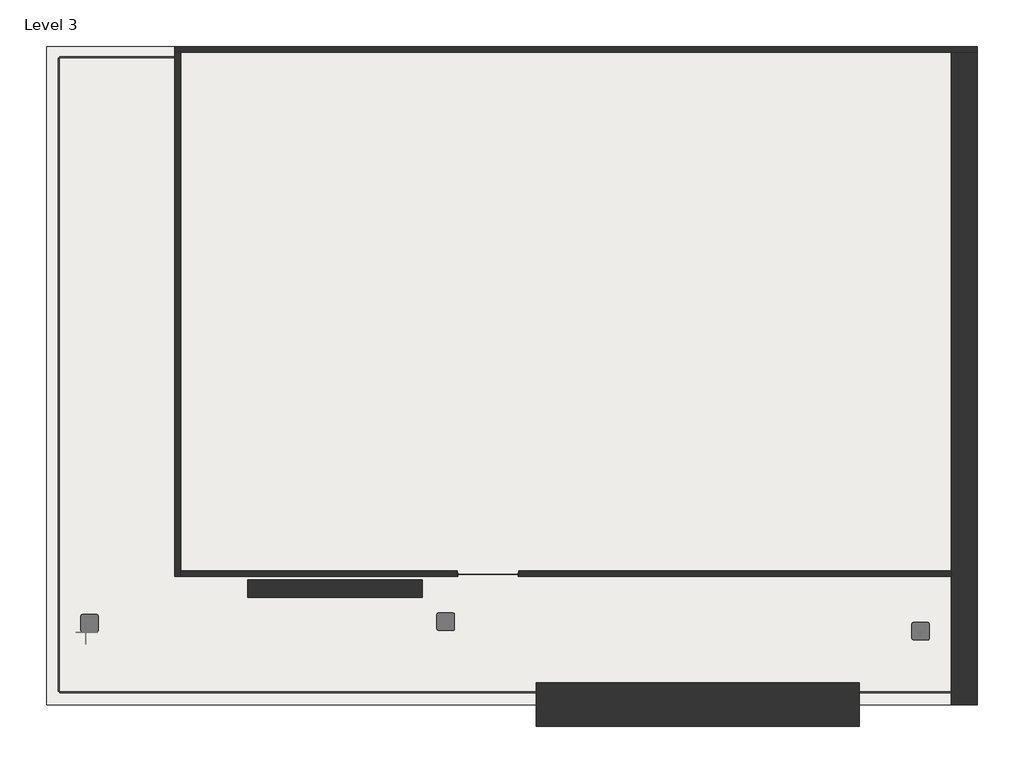
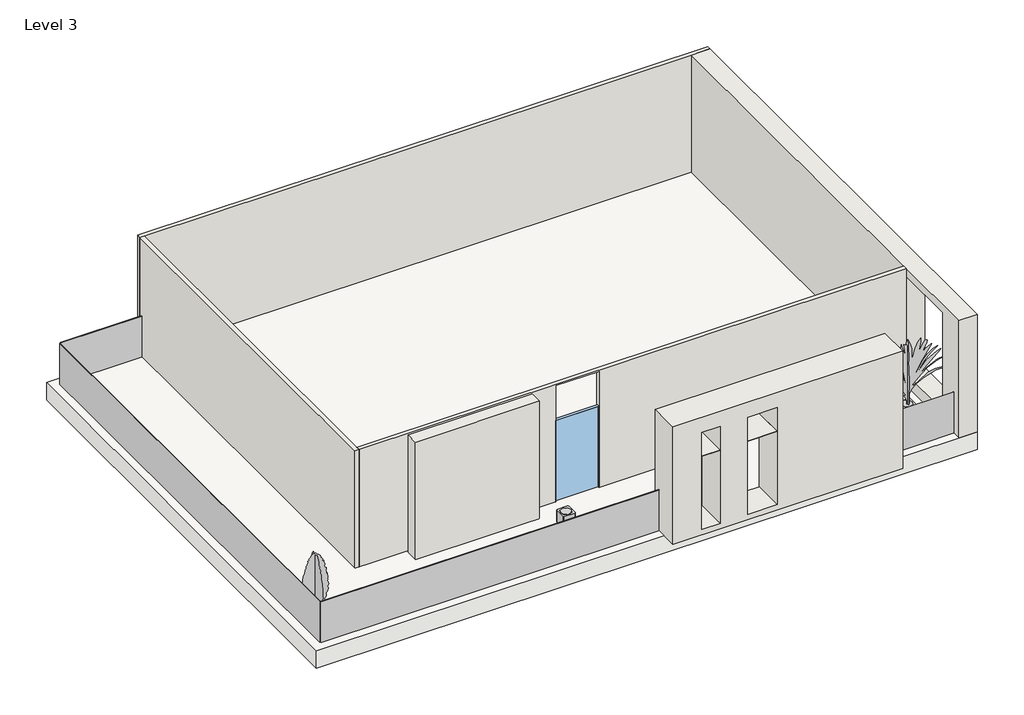
# One storey, incomplete: 6 walls, 4 plates, 3 proxies, 2 geographic elements, 1 slab, 1 window.
"""IFC4 building model written with IfcOpenShell, lengths in millimetres."""

from ifc_helpers import new_model, si_unit, frame, origin, place, context, project, spatial, polyline, outline, extrude, faceted_brep, transform, mapped, element, save
from components import proxy_13b82c07, rpc_tree_conifer_chinese_juniper_7_5155a079, rpc_tree_tropical_0177ab4a, system_panel_glazed_7ce5a3c2, system_panel_glazed_6867f845, system_panel_glazed_ba49168f, system_panel_glazed_c41ca4f4, window_2382273a

model = new_model("IFC4")

# Units and contexts
model_context = context("Model", 3, world=origin())
ifc_project = project(units=[si_unit("LENGTHUNIT", "METRE", prefix="MILLI")], contexts=[model_context])

# Site, building, storey
site = spatial("IfcSite", under=ifc_project)
building = spatial("IfcBuilding", under=site)
storey = spatial("IfcBuildingStorey", under=building, Name="Level 3", Elevation=6096.0)

# Proxies
placement = place(None, origin())
proxy_shape = proxy_13b82c07(model_context)
element("IfcBuildingElementProxy", 1, Name="Air Conditioner-Outside Unit : 33\" x 24\" x 24\"", ObjectType="Air Conditioner-Outside Unit : 33\" x 24\" x 24\"", at=placement, inside=storey, context=model_context, shape_type="MappedRepresentation", body=[
    mapped(proxy_shape, transform((-24603.5874719, -2613.1632813, 7010.4), x_axis=(1.0, 0.0, 0.0), y_axis=(0.0, 1.0, 0.0), z_axis=(0.0, 0.0, 1.0))),
])
element("IfcBuildingElementProxy", 2, Name="Air Conditioner-Outside Unit : 33\" x 24\" x 24\"", ObjectType="Air Conditioner-Outside Unit : 33\" x 24\" x 24\"", at=placement, inside=storey, context=model_context, shape_type="MappedRepresentation", body=[
    mapped(proxy_shape, transform((4377.8125281, -2892.5632813, 7010.4), x_axis=(1.0, 0.0, 0.0), y_axis=(0.0, 1.0, 0.0), z_axis=(0.0, 0.0, 1.0))),
])
element("IfcBuildingElementProxy", 3, Name="Air Conditioner-Outside Unit : 33\" x 24\" x 24\"", ObjectType="Air Conditioner-Outside Unit : 33\" x 24\" x 24\"", at=placement, inside=storey, context=model_context, shape_type="MappedRepresentation", body=[
    mapped(proxy_shape, transform((-12182.9874719, -2562.3632813, 7010.4), x_axis=(1.0, 0.0, 0.0), y_axis=(0.0, 1.0, 0.0), z_axis=(0.0, 0.0, 1.0))),
])

# Geographic elements
rpc_tree_conifer_chinese_juniper_7_shape = rpc_tree_conifer_chinese_juniper_7_5155a079(model_context)
element("IfcGeographicElement", 4, ObjectType="RPC Tree - Conifer : Chinese Juniper - 7'", at=placement, inside=storey, context=model_context, shape_type="MappedRepresentation", body=[
    mapped(rpc_tree_conifer_chinese_juniper_7_shape, transform((-24730.784143, -2943.3632813, 7010.4), x_axis=(1.0, 0.0, 0.0), y_axis=(0.0, 1.0, 0.0), z_axis=(0.0, 0.0, 1.0))),
])
rpc_tree_tropical_shape = rpc_tree_tropical_0177ab4a(model_context)
element("IfcGeographicElement", 5, ObjectType="RPC Tree - Tropical", at=placement, inside=storey, context=model_context, shape_type="MappedRepresentation", body=[
    mapped(rpc_tree_tropical_shape, transform((4377.8125281, -2943.3632813, 7010.4), x_axis=(1.0, 0.0, 0.0), y_axis=(0.0, 1.0, 0.0), z_axis=(0.0, 0.0, 1.0))),
])

# Plates
system_panel_glazed_shape = system_panel_glazed_7ce5a3c2(model_context)
element("IfcPlate", 6, ObjectType="System Panel : Glazed", at=placement, inside=storey, context=model_context, shape_type="MappedRepresentation", body=[
    mapped(system_panel_glazed_shape, transform((3844.4125281, -5000.7632813, 7010.4), x_axis=(-1.0, 0.0, 0.0), y_axis=(0.0, -1.0, 0.0), z_axis=(0.0, 0.0, 1.0))),
])
system_panel_glazed_2_shape = system_panel_glazed_6867f845(model_context)
element("IfcPlate", 7, ObjectType="System Panel : Glazed", at=placement, inside=storey, context=model_context, shape_type="MappedRepresentation", body=[
    mapped(system_panel_glazed_2_shape, transform((-17339.1874719, -5000.7632813, 7010.4), x_axis=(-1.0, 0.0, 0.0), y_axis=(0.0, -1.0, 0.0), z_axis=(0.0, 0.0, 1.0))),
])
system_panel_glazed_3_shape = system_panel_glazed_ba49168f(model_context)
element("IfcPlate", 8, ObjectType="System Panel : Glazed", at=placement, inside=storey, context=model_context, shape_type="MappedRepresentation", body=[
    mapped(system_panel_glazed_3_shape, transform((-25644.9874719, 6048.2367187, 7010.4), x_axis=(0.0, 1.0, 0.0), y_axis=(-1.0, 0.0, 0.0), z_axis=(0.0, 0.0, 1.0))),
])
system_panel_glazed_4_shape = system_panel_glazed_c41ca4f4(model_context)
element("IfcPlate", 9, ObjectType="System Panel : Glazed", at=placement, inside=storey, context=model_context, shape_type="MappedRepresentation", body=[
    mapped(system_panel_glazed_4_shape, transform((-23638.3874719, 17097.2367187, 7010.4), x_axis=(1.0, 0.0, 0.0), y_axis=(0.0, 1.0, 0.0), z_axis=(0.0, 0.0, 1.0))),
])

# Slab
element("IfcSlab", 10, ObjectType="Generic - 3'", at=placement, inside=storey, context=model_context, shape_type="SweptSolid", body=[
    extrude(outline(polyline([(-26102.1874719, -5457.9632813), (-26102.1874719, 17503.6367187), (6359.0125281, 17503.6367187), (6359.0125281, -5457.9632813), (-26102.1874719, -5457.9632813)])), frame((0.0, 0.0, 6096.0), z_axis=(0.0, 0.0, 1.0), x_axis=(1.0, 0.0, 0.0)), (0.0, 0.0, 1.0), 914.4),
])

# Walls
element("IfcWall", 11, ObjectType="Generic - 3'", at=placement, inside=storey, context=model_context, shape_type="Brep", body=[
    faceted_brep([(5444.6125281, 17300.4367187, 7010.4), (5444.6125281, -784.3632813, 7010.4), (5444.6125281, -987.5632813, 7010.4), (5444.6125281, -5457.9632813, 7010.4), (5444.6125281, -5457.9632813, 13106.4), (5444.6125281, -987.5632813, 13106.4), (5444.6125281, -784.3632813, 13106.4), (5444.6125281, 17300.4367187, 13106.4), (5444.6125281, -4035.5632813, 12658.887938), (5444.6125281, -4035.5632813, 7629.687938), (5444.6125281, -987.5632813, 7629.687938), (5444.6125281, -987.5632813, 12658.887938), (6359.0125281, 17300.4367187, 7010.4), (6359.0125281, 17300.4367187, 13106.4), (6359.0125281, -5457.9632813, 13106.4), (6359.0125281, -5457.9632813, 7010.4), (6359.0125281, -4035.5632813, 12658.887938), (6359.0125281, -987.5632813, 12658.887938), (6359.0125281, -987.5632813, 7629.687938), (6359.0125281, -4035.5632813, 7629.687938)], [[[0, 1, 2, 3, 4, 5, 6, 7], [8, 9, 10, 11]], [[12, 13, 14, 15], [16, 17, 18, 19]], [[0, 7, 13, 12]], [[3, 2, 1, 0, 12, 15]], [[4, 3, 15, 14]], [[7, 6, 5, 4, 14, 13]], [[9, 8, 16, 19]], [[10, 9, 19, 18]], [[8, 11, 17, 16]], [[11, 10, 18, 17]]]),
])
element("IfcWall", 12, ObjectType="Generic - 3' gray", at=placement, inside=storey, context=model_context, shape_type="SweptSolid", body=[
    extrude(outline(polyline([(7010.4, 2244.2125281), (13106.4, 2244.2125281), (13106.4, -9033.3874719), (7010.4, -9033.3874719), (7010.4, 2244.2125281)]), holes=[polyline([(12325.7308744, -6716.0306948), (11106.5308744, -6716.0306948), (11106.5308744, -7630.4306948), (12325.7308744, -7630.4306948), (12325.7308744, -6716.0306948)]), polyline([(7296.5308744, -7630.4306948), (11081.1308744, -7630.4306948), (11081.1308744, -6716.0306948), (7296.5308744, -6716.0306948), (7296.5308744, -7630.4306948)]), polyline([(12325.7308744, -3924.8577662), (11106.5308744, -3924.8577662), (11106.5308744, -5371.4183212), (12325.7308744, -5371.4183212), (12325.7308744, -3924.8577662)]), polyline([(7296.5308744, -5371.4183212), (11081.1308744, -5371.4183212), (11081.1308744, -3924.8577662), (7296.5308744, -3924.8577662), (7296.5308744, -5371.4183212)])]), frame((0.0, -6219.9632813, 0.0), z_axis=(0.0, 1.0, 0.0), x_axis=(0.0, 0.0, 1.0)), (0.0, 0.0, 1.0), 1524.0),
])
element("IfcWall", 13, ObjectType="Generic - 8\"", at=placement, inside=storey, context=model_context, shape_type="Brep", body=[
    faceted_brep([(-21631.7874719, 17300.4367187, 7010.4), (-21428.5874719, 17300.4367187, 7010.4), (5444.6125281, 17300.4367187, 7010.4), (6359.0125281, 17300.4367187, 7010.4), (6359.0125281, 17300.4367187, 13106.4), (5444.6125281, 17300.4367187, 13106.4), (-21428.5874719, 17300.4367187, 13106.4), (-21631.7874719, 17300.4367187, 13106.4), (-21631.7874719, 17503.6367187, 7010.4), (-21631.7874719, 17503.6367187, 13106.4), (6359.0125281, 17503.6367187, 13106.4), (6359.0125281, 17503.6367187, 7010.4)], [[[0, 1, 2, 3, 4, 5, 6, 7]], [[8, 9, 10, 11]], [[3, 2, 1, 0, 8, 11]], [[7, 6, 5, 4, 10, 9]], [[0, 7, 9, 8]], [[4, 3, 11, 10]]]),
])
element("IfcWall", 14, ObjectType="Generic - 8\"", at=placement, inside=storey, context=model_context, shape_type="Brep", body=[
    faceted_brep([(-21428.5874719, -987.5632813, 7010.4), (-21428.5874719, -784.3632813, 7010.4), (-21428.5874719, 17300.4367187, 7010.4), (-21428.5874719, 17300.4367187, 13106.4), (-21428.5874719, -784.3632813, 13106.4), (-21428.5874719, -987.5632813, 13106.4), (-21631.7874719, -987.5632813, 7010.4), (-21631.7874719, -987.5632813, 13106.4), (-21631.7874719, 17300.4367187, 13106.4), (-21631.7874719, 17300.4367187, 7010.4)], [[[0, 1, 2, 3, 4, 5]], [[6, 7, 8, 9]], [[2, 1, 0, 6, 9]], [[5, 4, 3, 8, 7]], [[0, 5, 7, 6]], [[3, 2, 9, 8]]]),
])
element("IfcWall", 15, ObjectType="Generic - 8\"", at=placement, inside=storey, context=model_context, shape_type="Brep", body=[
    faceted_brep([(-21428.5874719, -784.3632813, 13106.4), (5444.6125281, -784.3632813, 13106.4), (5444.6125281, -784.3632813, 7010.4), (-9642.9874719, -784.3632813, 7010.4), (-9642.9874719, -784.3632813, 13045.0483945), (-11776.5874719, -784.3632813, 13045.0483945), (-11776.5874719, -784.3632813, 7010.4), (-21428.5874719, -784.3632813, 7010.4), (5444.6125281, -987.5632813, 13106.4), (-21428.5874719, -987.5632813, 13106.4), (-21428.5874719, -987.5632813, 7010.4), (-11776.5874719, -987.5632813, 7010.4), (-11776.5874719, -987.5632813, 13045.0483945), (-9642.9874719, -987.5632813, 13045.0483945), (-9642.9874719, -987.5632813, 7010.4), (5444.6125281, -987.5632813, 7010.4), (5444.6125281, -987.5632813, 7629.687938), (5444.6125281, -987.5632813, 12658.887938)], [[[0, 1, 2, 3, 4, 5, 6, 7]], [[8, 9, 10, 11, 12, 13, 14, 15, 16, 17]], [[10, 7, 6, 11]], [[3, 2, 15, 14]], [[1, 0, 9, 8]], [[0, 7, 10, 9]], [[11, 6, 5, 12]], [[3, 14, 13, 4]], [[12, 5, 4, 13]], [[15, 2, 1, 8, 17, 16]]]),
])
element("IfcWall", 16, ObjectType="Generic -2", at=placement, inside=storey, context=model_context, shape_type="SweptSolid", body=[
    extrude(outline(polyline([(-12995.7874719, -1724.1632813), (-19091.7874719, -1724.1632813), (-19091.7874719, -1114.5632813), (-12995.7874719, -1114.5632813), (-12995.7874719, -1724.1632813)])), frame((0.0, 0.0, 7010.4), z_axis=(0.0, 0.0, 1.0), x_axis=(1.0, 0.0, 0.0)), (0.0, 0.0, 1.0), 6106.1211964),
])

# Window
window_shape = window_2382273a(model_context)
element("IfcWindow", 17, ObjectType="Instance - Fixed : 24\" x 48\"", at=placement, inside=storey, context=model_context, shape_type="MappedRepresentation", body=[
    mapped(window_shape, transform((-10747.8874719, -885.9632813, 6067.855451), x_axis=(-1.0, 0.0, 0.0), y_axis=(0.0, -1.0, 0.0), z_axis=(0.0, 0.0, 1.0))),
])

save(model, "model.ifc")

# Revit data of these elements
# Type "Air Conditioner-Outside Unit : 33\" x 24\" x 24\""
#   Assembly Code = "D3030"
#   Depth = 2' - 0"
#   Height = 2' - 0"
#   Width = 2' - 0"
#   Air Conditioner Material = Steel, Paint Finish, Dark Gray, Matte
#   Default Elevation = 0
# Type "RPC Tree - Conifer : Chinese Juniper - 7'"
#   built-in parameter 1005198 = "{2, 15},{39, RPC-16-FUM3-UUQ0-UBF0-N000-ST1L-LVER-AU},{1, 0},{1, 0},{2, 13},{1, 8},{5, Color},{1, 0},{1, 0},{3, 0.8},{3, 0.8},{3, 0.8},{1, 8},{7, BBoxMin},{1, 0},{1, 0},{1, 0},{1, 0},{1, 0},{1, 8},{7, BBoxMax},{1, 0},{1, 0},{1, 0},{1, 0},{1, 0},{2, 11},{9, RPCTypeId},{1, 0},{1, 0},{39, RPC-16-FUM3-UUQ0-UBF0-N000-ST1L-LVER-AU},{1, 6},{14, RPCPlantHeight},{1, 0},{1, 0},{1, 7},{2, 11},{7, keyword},{1, 0},{1, 0},{34, :RPCs:Trees [General]:Geometry:RPC},{2, 11},{8, category},{1, 0},{1, 0},{15, Trees [General]},{2, 11},{12, LocalizedUID},{1, 0},{1, 0},{15, Chinese Juniper},{2, 14},{6, Height},{1, 0},{1, 0},{1, 7},{1, 2},{16, Cast Reflections},{1, 0},{1, 0},{1, 0},{1, 2},{12, Cast Shadows},{1, 0},{1, 0},{1, 1},{1, 2},{9, Lock View},{1, 0},{1, 0},{1, 0},{1, 4},{5, ViewC},{1, 0},{1, 0},{1, 0},{21, assetlibrary_base.fbx},{1, 5},"
#   built-in parameter 1005195 = "RPC-16-FUM3-UUQ0-UBF0-N000-ST1L-LVER-AU"
#   Type Comments = "Chinese Juniper"
#   Assembly Code = "G2050500"
#   Height = 10' - 0"
#   Description = (empty or 0)
#   Default Elevation = 0
# Type "RPC Tree - Tropical"
#   built-in parameter 1005198 = "{2, 15},{39, RPC-16-G2M6-EAFX-C5H6-W000-ST1L-LVER-AU},{1, 0},{1, 0},{2, 13},{1, 8},{5, Color},{1, 0},{1, 0},{3, 0.8},{3, 0.8},{3, 0.8},{1, 8},{7, BBoxMin},{1, 0},{1, 0},{1, 0},{1, 0},{1, 0},{1, 8},{7, BBoxMax},{1, 0},{1, 0},{1, 0},{1, 0},{1, 0},{2, 11},{9, RPCTypeId},{1, 0},{1, 0},{39, RPC-16-G2M6-EAFX-C5H6-W000-ST1L-LVER-AU},{1, 6},{14, RPCPlantHeight},{1, 0},{1, 0},{2, 13},{2, 11},{7, keyword},{1, 0},{1, 0},{35, :RPCs:Trees [Tropical]:Geometry:RPC},{2, 11},{8, category},{1, 0},{1, 0},{16, Trees [Tropical]},{2, 11},{12, LocalizedUID},{1, 0},{1, 0},{15, Traveler's Palm},{2, 14},{6, Height},{1, 0},{1, 0},{2, 13},{1, 2},{16, Cast Reflections},{1, 0},{1, 0},{1, 0},{1, 2},{12, Cast Shadows},{1, 0},{1, 0},{1, 1},{1, 2},{9, Lock View},{1, 0},{1, 0},{1, 0},{1, 4},{5, ViewC},{1, 0},{1, 0},{1, 0},{21, assetlibrary_base.fbx},{1, 5},"
#   built-in parameter 1005195 = "RPC-16-G2M6-EAFX-C5H6-W000-ST1L-LVER-AU"
#   Assembly Code = "G2050500"
#   Height = 13' - 0"
#   Plan Symbol = element 321958
#   Default Elevation = 0
# Type "System Panel : Glazed"
#   Construction Type Id = "GSP4R"
#   Analytic Construction = "1/8 in Pilkington single glazing"
#   Visual Light Transmittance = 0.9
#   Solar Heat Gain Coefficient = 0.86
#   Heat Transfer Coefficient (U) = 1.18115 BTU/(h·ft²·°F)
# Type "Generic - 3'"
#   Assembly Code = "B1010"
#   Function = 0
#   Layers, outside or top first: 3' - 0" "Parking Stripe" (function 1)
# Type "Generic - 3'"
#   Assembly Code = "B2010"
#   Layers, outside or top first: 3' - 0" "Parking Stripe" (function 1)
# Type "Generic - 3' gray"
#   Assembly Code = "B2010"
#   Layers, outside or top first: 5' - 0" "Concrete, Lightweight" (function 1)
# Type "Generic - 8\""
#   Assembly Code = "B2010"
#   Layers, outside or top first: 0' - 8" no material (function 1)
# Type "Generic -2"
#   Assembly Code = "B2010"
#   Layers, outside or top first: 2' - 0" "Plywood, Sheathing" (function 1)
# Type "Instance - Fixed : 24\" x 48\""
#   Type Mark = "10"
#   Construction Type Id = "GSP4R"
#   Assembly Code = "B2020100"
#   Analytic Construction = "1/8 in Pilkington single glazing"
#   Visual Light Transmittance = 0.9
#   Thermal Resistance (R) = 0.8466 (h·ft²·°F)/BTU
#   Solar Heat Gain Coefficient = 0.86
#   Heat Transfer Coefficient (U) = 1.1812 BTU/(h·ft²·°F)
#   Height [instance default] = 4' - 0"
#   Default Sill Height = 3' - 0"
#   Width [instance default] = 2' - 0"
#   Window Inset = 0' - 2"
#   Define Thermal Properties by = 1
#   Glass Pane Material = Glass
#   Sash Material = Iron, Ductile
#   Wall Closure = (empty or 0)
# Element 1 (IfcBuildingElementProxy, "Air Conditioner-Outside Unit : 33\" x 24\" x 24\"")
#   Mark = "4"
#   Phase Created = New Construction
#   Materials on its faces: "Steel, Paint Finish, Dark Gray, Matte"
# Element 2 (IfcBuildingElementProxy, "Air Conditioner-Outside Unit : 33\" x 24\" x 24\"")
#   Mark = "5"
#   Phase Created = New Construction
#   Materials on its faces: "Steel, Paint Finish, Dark Gray, Matte"
# Element 3 (IfcBuildingElementProxy, "Air Conditioner-Outside Unit : 33\" x 24\" x 24\"")
#   Mark = "6"
#   Phase Created = New Construction
#   Materials on its faces: "Steel, Paint Finish, Dark Gray, Matte"
# Element 4 (IfcGeographicElement, "RPC Tree - Conifer : Chinese Juniper - 7'")
#   Phase Created = New Construction
# Element 5 (IfcGeographicElement, "RPC Tree - Tropical")
#   Phase Created = New Construction
# Elements 6, 7, 8, 9 (IfcPlate, "System Panel : Glazed")
#   Phase Created = New Construction
#   Materials on its faces: "Glass"
# Element 10 (IfcSlab, "Generic - 3'")
#   built-in parameter 1001955 = 3.14159 (stored number, unit not read)
#   Height Offset From Level = 3' - 0"
#   Phase Created = New Construction
#   Materials on its faces: "Parking Stripe"
# Element 11 (IfcWall, "Generic - 3'")
#   built-in parameter 1001111 = 3' - 0"
#   Top Offset = 0' - 0"
#   Base Offset = 3' - 0"
#   Unconnected Height = 20' - 0"
#   wall height = 20' - 0"
#   Phase Created = New Construction
#   Base Constraint = Level 3
#   Materials on its faces: "Parking Stripe", "Default Wall"
# Element 12 (IfcWall, "Generic - 3' gray")
#   built-in parameter 1001111 = 3' - 0"
#   Top Offset = 0' - 0"
#   Base Offset = 3' - 0"
#   Unconnected Height = 20' - 0"
#   wall height = 20' - 0"
#   Phase Created = New Construction
#   Base Constraint = Level 3
#   Materials on its faces: "Concrete, Lightweight"
# Element 13 (IfcWall, "Generic - 8\"")
#   built-in parameter 1001111 = 3' - 0"
#   Top Offset = 0' - 0"
#   Base Offset = 3' - 0"
#   Unconnected Height = 20' - 0"
#   wall height = 20' - 0"
#   Phase Created = New Construction
#   Base Constraint = Level 3
#   Materials on its faces: "Default Wall", "Parking Stripe"
# Elements 14, 15 (IfcWall, "Generic - 8\"")
#   built-in parameter 1001111 = 3' - 0"
#   Top Offset = 0' - 0"
#   Base Offset = 3' - 0"
#   Unconnected Height = 20' - 0"
#   wall height = 20' - 0"
#   Phase Created = New Construction
#   Base Constraint = Level 3
#   Materials on its faces: "Default Wall"
# Element 16 (IfcWall, "Generic -2")
#   built-in parameter 1001111 = 3' - 0"
#   Top Offset = 0' - 0"
#   Base Offset = 3' - 0"
#   Unconnected Height = 20' - 0.39847"
#   wall height = 20' - 0.39847"
#   Phase Created = New Construction
#   Base Constraint = Level 3
#   Materials on its faces: "Plywood, Sheathing"
# Element 17 (IfcWindow, "Instance - Fixed : 24\" x 48\"")
#   Mark = "3"
#   Width = 7' - 0"
#   Height = 14' - 0"
#   Phase Created = New Construction
#   Materials on its faces: "Iron, Ductile", "Glass"
# Materials
#   "Steel, Paint Finish, Dark Gray, Matte": class "Metal", colour RGB 98 98 98, transparency 0, Description = "Steel, paint finish, dark gray, matte", Cost = 0
#   "Parking Stripe": class "Paint", colour RGB 250 250 91, transparency 0, Cost = 0
#   "Concrete, Lightweight": class "Concrete", colour RGB 142 141 140, transparency 0, Description = "Lightweight concrete", Cost = 0
#   "Plywood, Sheathing": class "Wood", colour RGB 212 179 113, transparency 0, Description = "Plywood, sheathing grade", Cost = 0
#   "Glass": class "Glass", colour RGB 0 128 192, transparency 0.75, Description = "Soda Lime Glass", Cost = 0
#   "Iron, Ductile": class "Metal", colour RGB 0 0 0, transparency 0, Description = "Ductile cast iron", Cost = 0
#   "Default Wall": colour RGB 128 128 128, transparency 0
